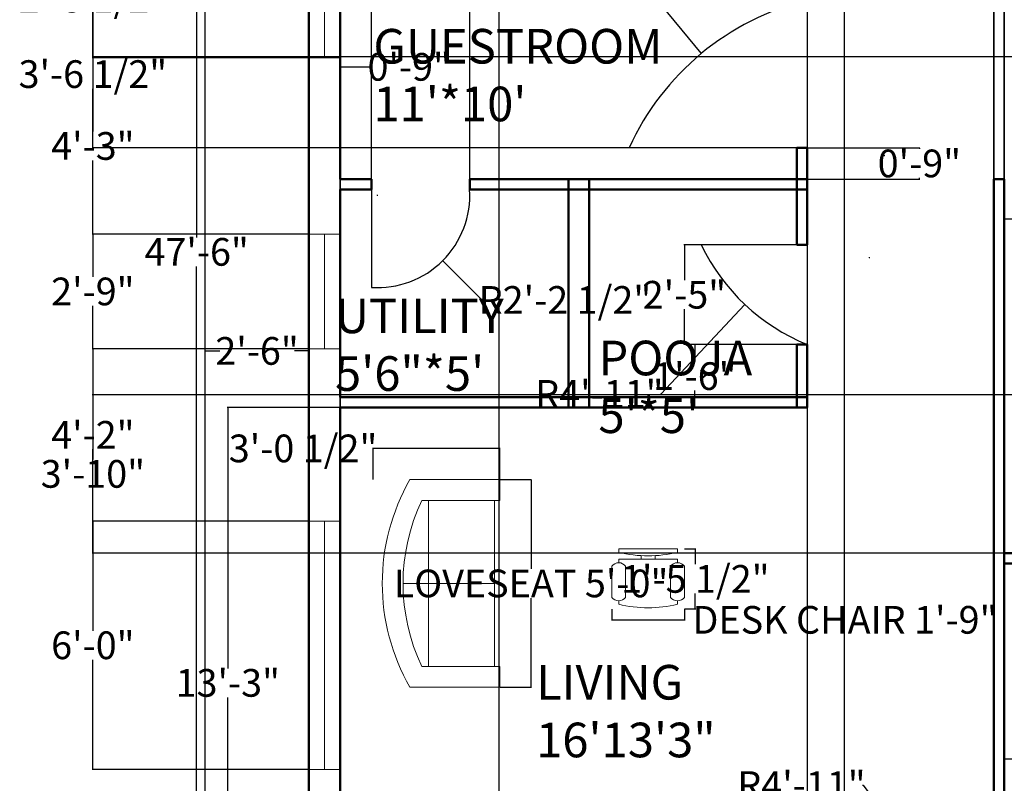
# Model space of a CAD drawing. Units: inches. Extents: x 3437 to 3994, y 3379 to 4084.
# Tile 2 of 6: x 3437 to 3722, y 3555 to 3776. Entities that reach past the tile are written whole.
import ezdxf

# ---------------------------------------------------------------- set-up
doc = ezdxf.new("R2010")
doc.units = ezdxf.units.IN
doc.header["$MEASUREMENT"] = 0
for name, color, linetype, lineweight in [('A-ANNO-DIMS', 2, 'Continuous', 18), ('A-AREA-IDEN', 7, 'Continuous', 25), ('A-DOOR', 3, 'Continuous', 25), ('A-FLOR-CASE', 8, 'Continuous', 25), ('A-FLOR-STRS', 7, 'Continuous', 25), ('A-FURN', 8, 'Continuous', 18), ('A-GLAZ', 4, 'Continuous', 18), ('A-WALL', 7, 'Continuous', 50), ('C-PROP', 3, 'Continuous', 25)]:
    doc.layers.add(name, color=color, linetype=linetype, lineweight=lineweight)
doc.styles.get("Standard").update_dxf_attribs({"font": 'arial.ttf'})
doc.dimstyles.get("Standard").update_dxf_attribs({"dimtxt": 8, "dimasz": 0.18, "dimexe": 0.18, "dimexo": 0.0625, "dimgap": 0.09, "dimtad": 0, "dimtih": 1, "dimtoh": 1, "dimdec": 0, "dimzin": 0, "dimdsep": 46, "dimlunit": 3, "dimtxsty": 'Standard', "dimcen": 0.09, "dimadec": 0, "dimazin": 0, "dimtfac": 1, "dimtdec": 0, "dimtofl": 0, "dimtmove": 0, "dimatfit": 3, "dimfxl": 1, "dimtolj": 1, "dimtzin": 0, "dimarcsym": 0})

# ---------------------------------------------------------------- blocks, each defined once
blk = doc.blocks.new('Sofa - Roundback Loveseat 5 ft.')
for p, q in [((0, -32.44198), (0, -5.99998)), ((-24, -33.99998), (-24, -11.46958)), ((-23.9998, -13.38178), (23.99986, -13.38178)), ((24.00004, -33.99998), (24.00004, -11.46958)), ((-24, -32.44198), (24.00004, -32.44198))]:
    blk.add_line(p, q)
for points in [[(-24, -33.99998), (-30, -33.99998), (-30, -7.99998)], [(30.00004, -7.99998), (30.00004, -33.99998), (24.00004, -33.99998)]]:
    blk.add_lwpolyline(points)
for centre, radius, start, end in [((0, -60.24998), 60.24998, 60.13715, 119.8628), ((0, -61.38438), 55.38444, 64.32083, 115.6792)]:
    blk.add_arc(centre, radius, start, end)
blk = doc.blocks.new('Chair - Desk')
for p, q in [((-8.5, 0), (-8.5, -1)), ((-8.5, 0), (8.5, 0)), ((8.5, 0), (8.5, -1)), ((-2, -3), (-2, -1.9355)), ((2, -1.9576), (2, -3)), ((-10.5, -5), (-10.5, -14)), ((-8.5, -3), (-8.5, -4)), ((-8.5, -3), (8.5, -3)), ((-6.5, -14), (-6.5, -5)), ((6.5, -5), (6.5, -14)), ((8.5, -3), (8.5, -4)), ((10.5, -14), (10.5, -5)), ((-8.5, -15), (-8.5, -16)), ((8.5, -15), (8.5, -16))]:
    blk.add_line(p, q)
for centre, radius, start, end in [((0, 34.625), 36.625, 256.5803, 283.4197), ((-8.5, -6.5), 2.5, 36.8699, 143.1301), ((8.5, -6.5), 2.5, 36.8699, 143.1301), ((-8.5, -12.5), 2.5, 216.8699, 323.1301), ((8.5, -12.5), 2.5, 216.8699, 323.1301), ((0, 19.625), 36.625, 256.5803, 283.4197)]:
    blk.add_arc(centre, radius, start, end)
blk = doc.blocks.new('*D12')
at = {"layer": 'A-ANNO-DIMS', "color": 0, "lineweight": -2, "transparency": 16777216}
for p, q in [((3491.02, 3671.63), (3491.02, 3680.21)), ((3491.2, 3680.03), (3495.23, 3680.03)), ((3520.84, 3680.03), (3516.82, 3680.03)), ((3521.02, 3671.63), (3521.02, 3680.21))]:
    blk.add_line(p, q, dxfattribs=at)
at = {"layer": 'A-ANNO-DIMS', "color": 0, "transparency": 16777216}
for points in [[(3491.2, 3680.06), (3491.2, 3680), (3491.02, 3680.03)], [(3520.84, 3680.06), (3520.84, 3680), (3521.02, 3680.03)]]:
    blk.add_solid(points, dxfattribs=at)
at = {"layer": 'Defpoints', "color": 0, "transparency": 16777216}
for p in [(3491.02, 3680.03), (3491.02, 3671.57), (3521.02, 3671.57)]:
    blk.add_point(p, dxfattribs=at)
at = {"layer": 'A-ANNO-DIMS', "color": 0, "transparency": 16777216, "insert": (3506.02, 3680.03), "char_height": 8, "attachment_point": 5}
blk.add_mtext('\\A1;2\'-6"', dxfattribs=at)
blk = doc.blocks.new('*D21')
at = {"layer": 'A-ANNO-DIMS', "color": 0, "lineweight": -2, "transparency": 16777216}
for p, q in [((3576.28, 3642.87), (3585.4, 3642.87)), ((3585.22, 3642.69), (3585.22, 3617.09)), ((3585.22, 3583.05), (3585.22, 3608.64)), ((3576.28, 3582.87), (3585.4, 3582.87))]:
    blk.add_line(p, q, dxfattribs=at)
at = {"layer": 'A-ANNO-DIMS', "color": 0, "transparency": 16777216}
for points in [[(3585.19, 3642.69), (3585.25, 3642.69), (3585.22, 3642.87)], [(3585.19, 3583.05), (3585.25, 3583.05), (3585.22, 3582.87)]]:
    blk.add_solid(points, dxfattribs=at)
at = {"layer": 'Defpoints', "color": 0, "transparency": 16777216}
for p in [(3576.22, 3642.87), (3585.22, 3642.87), (3576.22, 3582.87)]:
    blk.add_point(p, dxfattribs=at)
at = {"layer": 'A-ANNO-DIMS', "color": 0, "transparency": 16777216, "insert": (3585.22, 3612.87), "char_height": 8, "attachment_point": 5}
blk.add_mtext('\\A1;LOVESEAT 5\'-0"', dxfattribs=at)
blk = doc.blocks.new('*D22')
at = {"layer": 'A-ANNO-DIMS', "color": 0, "lineweight": -2, "transparency": 16777216}
for p, q in [((3539.55, 3651.87), (3539.37, 3651.87)), ((3539.55, 3642.93), (3539.55, 3652.05)), ((3576.04, 3651.87), (3539.73, 3651.87)), ((3576.22, 3642.93), (3576.22, 3652.05))]:
    blk.add_line(p, q, dxfattribs=at)
at = {"layer": 'A-ANNO-DIMS', "color": 0, "transparency": 16777216}
for points in [[(3539.73, 3651.9), (3539.73, 3651.84), (3539.55, 3651.87)], [(3576.04, 3651.9), (3576.04, 3651.84), (3576.22, 3651.87)]]:
    blk.add_solid(points, dxfattribs=at)
at = {"layer": 'Defpoints', "color": 0, "transparency": 16777216}
for p in [(3539.55, 3651.87), (3539.55, 3642.87), (3576.22, 3642.87)]:
    blk.add_point(p, dxfattribs=at)
at = {"layer": 'A-ANNO-DIMS', "color": 0, "transparency": 16777216, "insert": (3519.33, 3651.87), "char_height": 8, "attachment_point": 5}
blk.add_mtext('\\A1;3\'-0 1/2"', dxfattribs=at)
blk = doc.blocks.new('*D25')
at = {"layer": 'A-ANNO-DIMS', "color": 0, "lineweight": -2, "transparency": 16777216}
for p, q in [((3608.56, 3605.44), (3608.56, 3602.17)), ((3629.56, 3605.44), (3629.56, 3602.17)), ((3608.74, 3602.35), (3629.38, 3602.35)), ((3629.56, 3602.35), (3629.74, 3602.35))]:
    blk.add_line(p, q, dxfattribs=at)
at = {"layer": 'A-ANNO-DIMS', "color": 0, "transparency": 16777216}
for points in [[(3608.74, 3602.38), (3608.74, 3602.32), (3608.56, 3602.35)], [(3629.38, 3602.38), (3629.38, 3602.32), (3629.56, 3602.35)]]:
    blk.add_solid(points, dxfattribs=at)
at = {"layer": 'Defpoints', "color": 0, "transparency": 16777216}
for p in [(3608.56, 3605.5), (3629.56, 3605.5), (3629.56, 3602.35)]:
    blk.add_point(p, dxfattribs=at)
at = {"layer": 'A-ANNO-DIMS', "color": 0, "transparency": 16777216, "insert": (3675.97, 3602.35), "char_height": 8, "attachment_point": 5}
blk.add_mtext('\\A1;DESK CHAIR 1\'-9"', dxfattribs=at)
blk = doc.blocks.new('*D26')
at = {"layer": 'A-ANNO-DIMS', "color": 0, "lineweight": -2, "transparency": 16777216}
for p, q in [((3629.62, 3622.84), (3632.89, 3622.84)), ((3632.71, 3622.66), (3632.71, 3618.39)), ((3632.71, 3605.68), (3632.71, 3609.94)), ((3629.62, 3605.5), (3632.89, 3605.5))]:
    blk.add_line(p, q, dxfattribs=at)
at = {"layer": 'A-ANNO-DIMS', "color": 0, "transparency": 16777216}
for points in [[(3632.68, 3622.66), (3632.74, 3622.66), (3632.71, 3622.84)], [(3632.68, 3605.68), (3632.74, 3605.68), (3632.71, 3605.5)]]:
    blk.add_solid(points, dxfattribs=at)
at = {"layer": 'Defpoints', "color": 0, "transparency": 16777216}
for p in [(3629.56, 3622.84), (3632.71, 3622.84), (3629.56, 3605.5)]:
    blk.add_point(p, dxfattribs=at)
at = {"layer": 'A-ANNO-DIMS', "color": 0, "transparency": 16777216, "insert": (3632.71, 3614.17), "char_height": 8, "attachment_point": 5}
blk.add_mtext('\\A1;1\'-5 1/2"', dxfattribs=at)
blk = doc.blocks.new('*D28')
at = {"layer": 'A-ANNO-DIMS', "color": 0, "lineweight": -2, "transparency": 16777216}
for p, q in [((3520.96, 3993.64), (3488.39, 3993.64)), ((3488.57, 3993.46), (3488.57, 3712.81)), ((3488.57, 3423.82), (3488.57, 3704.46)), ((3520.96, 3423.64), (3488.39, 3423.64))]:
    blk.add_line(p, q, dxfattribs=at)
at = {"layer": 'A-ANNO-DIMS', "color": 0, "transparency": 16777216}
for points in [[(3488.54, 3993.46), (3488.6, 3993.46), (3488.57, 3993.64)], [(3488.54, 3423.82), (3488.6, 3423.82), (3488.57, 3423.64)]]:
    blk.add_solid(points, dxfattribs=at)
at = {"layer": 'Defpoints', "color": 0, "transparency": 16777216}
for p in [(3488.57, 3993.64), (3521.02, 3993.64), (3521.02, 3423.64)]:
    blk.add_point(p, dxfattribs=at)
at = {"layer": 'A-ANNO-DIMS', "color": 0, "transparency": 16777216, "insert": (3488.57, 3708.64), "char_height": 8, "attachment_point": 5}
blk.add_mtext('\\A1;47\'-6"', dxfattribs=at)
blk = doc.blocks.new('*D36')
at = {"layer": 'A-ANNO-DIMS', "color": 0, "lineweight": -2, "transparency": 16777216}
for p, q in [((3520.96, 3821.48), (3458.39, 3821.48)), ((3458.57, 3821.3), (3458.57, 3797.26)), ((3458.57, 3764.87), (3458.57, 3788.91)), ((3520.96, 3764.69), (3458.39, 3764.69))]:
    blk.add_line(p, q, dxfattribs=at)
at = {"layer": 'A-ANNO-DIMS', "color": 0, "transparency": 16777216}
for points in [[(3458.54, 3821.3), (3458.6, 3821.3), (3458.57, 3821.48)], [(3458.54, 3764.87), (3458.6, 3764.87), (3458.57, 3764.69)]]:
    blk.add_solid(points, dxfattribs=at)
at = {"layer": 'Defpoints', "color": 0, "transparency": 16777216}
for p in [(3521.02, 3821.48), (3458.57, 3764.69), (3521.02, 3764.69)]:
    blk.add_point(p, dxfattribs=at)
at = {"layer": 'A-ANNO-DIMS', "color": 0, "transparency": 16777216, "insert": (3458.57, 3793.09), "char_height": 8, "attachment_point": 5}
blk.add_mtext('\\A1;4\'-9"', dxfattribs=at)
blk = doc.blocks.new('*D37')
at = {"layer": 'A-ANNO-DIMS', "color": 0, "lineweight": -2, "transparency": 16777216}
for p, q in [((3520.96, 3764.69), (3458.39, 3764.69)), ((3458.57, 3764.51), (3458.57, 3743.41)), ((3458.57, 3713.95), (3458.57, 3735.05)), ((3520.96, 3713.77), (3458.39, 3713.77))]:
    blk.add_line(p, q, dxfattribs=at)
at = {"layer": 'A-ANNO-DIMS', "color": 0, "transparency": 16777216}
for points in [[(3458.54, 3764.51), (3458.6, 3764.51), (3458.57, 3764.69)], [(3458.54, 3713.95), (3458.6, 3713.95), (3458.57, 3713.77)]]:
    blk.add_solid(points, dxfattribs=at)
at = {"layer": 'Defpoints', "color": 0, "transparency": 16777216}
for p in [(3521.02, 3764.69), (3458.57, 3713.77), (3521.02, 3713.77)]:
    blk.add_point(p, dxfattribs=at)
at = {"layer": 'A-ANNO-DIMS', "color": 0, "transparency": 16777216, "insert": (3458.57, 3739.23), "char_height": 8, "attachment_point": 5}
blk.add_mtext('\\A1;4\'-3"', dxfattribs=at)
blk = doc.blocks.new('*D38')
at = {"layer": 'A-ANNO-DIMS', "color": 0, "lineweight": -2, "transparency": 16777216}
for p, q in [((3520.96, 3713.77), (3458.39, 3713.77)), ((3458.57, 3713.59), (3458.57, 3701.39)), ((3458.57, 3680.83), (3458.57, 3693.04)), ((3520.96, 3680.65), (3458.39, 3680.65))]:
    blk.add_line(p, q, dxfattribs=at)
at = {"layer": 'A-ANNO-DIMS', "color": 0, "transparency": 16777216}
for points in [[(3458.54, 3713.59), (3458.6, 3713.59), (3458.57, 3713.77)], [(3458.54, 3680.83), (3458.6, 3680.83), (3458.57, 3680.65)]]:
    blk.add_solid(points, dxfattribs=at)
at = {"layer": 'Defpoints', "color": 0, "transparency": 16777216}
for p in [(3521.02, 3713.77), (3458.57, 3680.65), (3521.02, 3680.65)]:
    blk.add_point(p, dxfattribs=at)
at = {"layer": 'A-ANNO-DIMS', "color": 0, "transparency": 16777216, "insert": (3458.57, 3697.21), "char_height": 8, "attachment_point": 5}
blk.add_mtext('\\A1;2\'-9"', dxfattribs=at)
blk = doc.blocks.new('*D39')
at = {"layer": 'A-ANNO-DIMS', "color": 0, "lineweight": -2, "transparency": 16777216}
for p, q in [((3520.96, 3680.65), (3458.39, 3680.65)), ((3458.57, 3680.47), (3458.57, 3659.88)), ((3458.57, 3631.08), (3458.57, 3651.67)), ((3520.96, 3630.9), (3458.39, 3630.9))]:
    blk.add_line(p, q, dxfattribs=at)
at = {"layer": 'A-ANNO-DIMS', "color": 0, "transparency": 16777216}
for points in [[(3458.54, 3680.47), (3458.6, 3680.47), (3458.57, 3680.65)], [(3458.54, 3631.08), (3458.6, 3631.08), (3458.57, 3630.9)]]:
    blk.add_solid(points, dxfattribs=at)
at = {"layer": 'Defpoints', "color": 0, "transparency": 16777216}
for p in [(3521.02, 3680.65), (3458.57, 3630.9), (3521.02, 3630.9)]:
    blk.add_point(p, dxfattribs=at)
at = {"layer": 'A-ANNO-DIMS', "color": 0, "transparency": 16777216, "insert": (3458.57, 3655.78), "char_height": 8, "attachment_point": 5}
blk.add_mtext('\\A1;4\'-2"', dxfattribs=at)
blk = doc.blocks.new('*D40')
at = {"layer": 'A-ANNO-DIMS', "color": 0, "lineweight": -2, "transparency": 16777216}
for p, q in [((3520.96, 3630.9), (3458.39, 3630.9)), ((3458.57, 3630.72), (3458.57, 3599.17)), ((3458.57, 3559.28), (3458.57, 3590.83)), ((3520.96, 3559.1), (3458.39, 3559.1))]:
    blk.add_line(p, q, dxfattribs=at)
at = {"layer": 'A-ANNO-DIMS', "color": 0, "transparency": 16777216}
for points in [[(3458.54, 3630.72), (3458.6, 3630.72), (3458.57, 3630.9)], [(3458.54, 3559.28), (3458.6, 3559.28), (3458.57, 3559.1)]]:
    blk.add_solid(points, dxfattribs=at)
at = {"layer": 'Defpoints', "color": 0, "transparency": 16777216}
for p in [(3521.02, 3630.9), (3458.57, 3559.1), (3521.02, 3559.1)]:
    blk.add_point(p, dxfattribs=at)
at = {"layer": 'A-ANNO-DIMS', "color": 0, "transparency": 16777216, "insert": (3458.57, 3595), "char_height": 8, "attachment_point": 5}
blk.add_mtext('\\A1;6\'-0"', dxfattribs=at)
blk = doc.blocks.new('*D46')
at = {"layer": 'A-ANNO-DIMS', "color": 0, "lineweight": -2, "transparency": 16777216}
for p, q in [((3576.02, 3426.7), (3576.02, 4056.27)), ((3576.2, 4056.09), (3635.57, 4056.09)), ((3721.84, 4056.09), (3662.48, 4056.09)), ((3722.02, 3426.7), (3722.02, 4056.27))]:
    blk.add_line(p, q, dxfattribs=at)
at = {"layer": 'A-ANNO-DIMS', "color": 0, "transparency": 16777216}
for points in [[(3576.2, 4056.12), (3576.2, 4056.06), (3576.02, 4056.09)], [(3721.84, 4056.12), (3721.84, 4056.06), (3722.02, 4056.09)]]:
    blk.add_solid(points, dxfattribs=at)
at = {"layer": 'Defpoints', "color": 0, "transparency": 16777216}
for p in [(3722.02, 4056.09), (3576.02, 3426.64), (3722.02, 3426.64)]:
    blk.add_point(p, dxfattribs=at)
at = {"layer": 'A-ANNO-DIMS', "color": 0, "transparency": 16777216, "insert": (3649.02, 4056.09), "char_height": 8, "attachment_point": 5}
blk.add_mtext('\\A1;12\'-2"', dxfattribs=at)
blk = doc.blocks.new('*D47')
at = {"layer": 'A-ANNO-DIMS', "color": 0, "lineweight": -2, "transparency": 16777216}
for p, q in [((3521.02, 3993.57), (3521.02, 3391.01)), ((3530.02, 3984.57), (3530.02, 3391.01)), ((3521.2, 3391.19), (3529.84, 3391.19)), ((3530.02, 3391.19), (3530.2, 3391.19))]:
    blk.add_line(p, q, dxfattribs=at)
at = {"layer": 'A-ANNO-DIMS', "color": 0, "transparency": 16777216}
for points in [[(3521.2, 3391.22), (3521.2, 3391.16), (3521.02, 3391.19)], [(3529.84, 3391.22), (3529.84, 3391.16), (3530.02, 3391.19)]]:
    blk.add_solid(points, dxfattribs=at)
at = {"layer": 'Defpoints', "color": 0, "transparency": 16777216}
for p in [(3521.02, 3993.64), (3530.02, 3984.64), (3530.02, 3391.19)]:
    blk.add_point(p, dxfattribs=at)
at = {"layer": 'A-ANNO-DIMS', "color": 0, "transparency": 16777216, "insert": (3540.93, 3391.19), "char_height": 8, "attachment_point": 5}
blk.add_mtext('\\A1;0\'-9"', dxfattribs=at)
blk = doc.blocks.new('*D48')
at = {"layer": 'A-ANNO-DIMS', "color": 0, "lineweight": -2, "transparency": 16777216}
for p, q in [((3722.02, 3861.57), (3722.02, 3391.01)), ((3719.02, 3858.57), (3719.02, 3391.01)), ((3719.2, 3391.19), (3721.84, 3391.19)), ((3722.02, 3391.19), (3722.2, 3391.19))]:
    blk.add_line(p, q, dxfattribs=at)
at = {"layer": 'A-ANNO-DIMS', "color": 0, "transparency": 16777216}
for points in [[(3719.2, 3391.22), (3719.2, 3391.16), (3719.02, 3391.19)], [(3721.84, 3391.22), (3721.84, 3391.16), (3722.02, 3391.19)]]:
    blk.add_solid(points, dxfattribs=at)
at = {"layer": 'Defpoints', "color": 0, "transparency": 16777216}
for p in [(3722.02, 3861.64), (3719.02, 3858.64), (3722.02, 3391.19)]:
    blk.add_point(p, dxfattribs=at)
at = {"layer": 'A-ANNO-DIMS', "color": 0, "transparency": 16777216, "insert": (3732.93, 3391.19), "char_height": 8, "attachment_point": 5}
blk.add_mtext('\\A1;0\'-3"', dxfattribs=at)
blk = doc.blocks.new('*D49')
at = {"layer": 'A-ANNO-DIMS', "color": 0, "lineweight": -2, "transparency": 16777216}
for p, q in [((3530.02, 3504.7), (3530.02, 4056.27)), ((3530.2, 4056.09), (3611.07, 4056.09)), ((3718.84, 4056.09), (3637.98, 4056.09)), ((3719.02, 3504.7), (3719.02, 4056.27))]:
    blk.add_line(p, q, dxfattribs=at)
at = {"layer": 'A-ANNO-DIMS', "color": 0, "transparency": 16777216}
for points in [[(3530.2, 4056.12), (3530.2, 4056.06), (3530.02, 4056.09)], [(3718.84, 4056.12), (3718.84, 4056.06), (3719.02, 4056.09)]]:
    blk.add_solid(points, dxfattribs=at)
at = {"layer": 'Defpoints', "color": 0, "transparency": 16777216}
for p in [(3719.02, 4056.09), (3530.02, 3504.64), (3719.02, 3504.64)]:
    blk.add_point(p, dxfattribs=at)
at = {"layer": 'A-ANNO-DIMS', "color": 0, "transparency": 16777216, "insert": (3624.52, 4056.09), "char_height": 8, "attachment_point": 5}
blk.add_mtext('\\A1;15\'-9"', dxfattribs=at)
blk = doc.blocks.new('*D50')
at = {"layer": 'A-ANNO-DIMS', "color": 0, "lineweight": -2, "transparency": 16777216}
for p, q in [((3529.96, 3663.64), (3497.39, 3663.64)), ((3497.57, 3663.46), (3497.57, 3588.31)), ((3497.57, 3504.82), (3497.57, 3579.96)), ((3529.96, 3504.64), (3497.39, 3504.64))]:
    blk.add_line(p, q, dxfattribs=at)
at = {"layer": 'A-ANNO-DIMS', "color": 0, "transparency": 16777216}
for points in [[(3497.54, 3663.46), (3497.6, 3663.46), (3497.57, 3663.64)], [(3497.54, 3504.82), (3497.6, 3504.82), (3497.57, 3504.64)]]:
    blk.add_solid(points, dxfattribs=at)
at = {"layer": 'Defpoints', "color": 0, "transparency": 16777216}
for p in [(3497.57, 3663.64), (3530.02, 3663.64), (3530.02, 3504.64)]:
    blk.add_point(p, dxfattribs=at)
at = {"layer": 'A-ANNO-DIMS', "color": 0, "transparency": 16777216, "insert": (3497.57, 3584.14), "char_height": 8, "attachment_point": 5}
blk.add_mtext('\\A1;13\'-3"', dxfattribs=at)
blk = doc.blocks.new('*D59')
at = {"layer": 'A-ANNO-DIMS', "color": 0, "lineweight": -2, "transparency": 16777216}
for p, q in [((3661.96, 3781.25), (3458.39, 3781.25)), ((3458.57, 3781.07), (3458.57, 3764.22)), ((3458.57, 3738.92), (3458.57, 3755.76)), ((3661.96, 3738.74), (3458.39, 3738.74))]:
    blk.add_line(p, q, dxfattribs=at)
at = {"layer": 'A-ANNO-DIMS', "color": 0, "transparency": 16777216}
for points in [[(3458.54, 3781.07), (3458.6, 3781.07), (3458.57, 3781.25)], [(3458.54, 3738.92), (3458.6, 3738.92), (3458.57, 3738.74)]]:
    blk.add_solid(points, dxfattribs=at)
at = {"layer": 'Defpoints', "color": 0, "transparency": 16777216}
for p in [(3662.02, 3781.25), (3458.57, 3738.74), (3662.02, 3738.74)]:
    blk.add_point(p, dxfattribs=at)
at = {"layer": 'A-ANNO-DIMS', "color": 0, "transparency": 16777216, "insert": (3458.57, 3759.99), "char_height": 8, "attachment_point": 5}
blk.add_mtext('\\A1;3\'-6 1/2"', dxfattribs=at)
blk = doc.blocks.new('*D60')
at = {"layer": 'A-ANNO-DIMS', "color": 0, "lineweight": -2, "transparency": 16777216}
for p, q in [((3539.11, 3729.7), (3539.11, 4056.27)), ((3539.29, 4056.09), (3567.31, 4056.09)), ((3567.49, 3729.7), (3567.49, 4056.27)), ((3567.49, 4056.09), (3567.67, 4056.09))]:
    blk.add_line(p, q, dxfattribs=at)
at = {"layer": 'A-ANNO-DIMS', "color": 0, "transparency": 16777216}
for points in [[(3539.29, 4056.12), (3539.29, 4056.06), (3539.11, 4056.09)], [(3567.31, 4056.12), (3567.31, 4056.06), (3567.49, 4056.09)]]:
    blk.add_solid(points, dxfattribs=at)
at = {"layer": 'Defpoints', "color": 0, "transparency": 16777216}
for p in [(3567.49, 4056.09), (3539.11, 3729.64), (3567.49, 3729.64)]:
    blk.add_point(p, dxfattribs=at)
at = {"layer": 'A-ANNO-DIMS', "color": 0, "transparency": 16777216, "insert": (3587.78, 4056.09), "char_height": 8, "attachment_point": 5}
blk.add_mtext('\\A1;2\'-4 1/2"', dxfattribs=at)
blk = doc.blocks.new('*D61')
at = {"layer": 'A-ANNO-DIMS', "color": 0, "lineweight": -2, "transparency": 16777216}
for p, q in [((3661.96, 3710.64), (3629.39, 3710.64)), ((3629.57, 3710.46), (3629.57, 3700.43)), ((3629.57, 3682.05), (3629.57, 3692.08)), ((3661.96, 3681.87), (3629.39, 3681.87))]:
    blk.add_line(p, q, dxfattribs=at)
at = {"layer": 'A-ANNO-DIMS', "color": 0, "transparency": 16777216}
for points in [[(3629.54, 3710.46), (3629.6, 3710.46), (3629.57, 3710.64)], [(3629.54, 3682.05), (3629.6, 3682.05), (3629.57, 3681.87)]]:
    blk.add_solid(points, dxfattribs=at)
at = {"layer": 'Defpoints', "color": 0, "transparency": 16777216}
for p in [(3629.57, 3710.64), (3662.02, 3710.64), (3662.02, 3681.87)]:
    blk.add_point(p, dxfattribs=at)
at = {"layer": 'A-ANNO-DIMS', "color": 0, "transparency": 16777216, "insert": (3629.57, 3696.25), "char_height": 8, "attachment_point": 5}
blk.add_mtext('\\A1;2\'-5"', dxfattribs=at)
blk = doc.blocks.new('*D66')
at = {"layer": 'A-ANNO-DIMS', "color": 0, "lineweight": -2, "transparency": 16777216}
for p, q in [((3871.96, 3667.39), (3458.39, 3667.39)), ((3458.57, 3667.21), (3458.57, 3648.69)), ((3458.57, 3621.82), (3458.57, 3640.34)), ((3871.96, 3621.64), (3458.39, 3621.64))]:
    blk.add_line(p, q, dxfattribs=at)
at = {"layer": 'A-ANNO-DIMS', "color": 0, "transparency": 16777216}
for points in [[(3458.54, 3667.21), (3458.6, 3667.21), (3458.57, 3667.39)], [(3458.54, 3621.82), (3458.6, 3621.82), (3458.57, 3621.64)]]:
    blk.add_solid(points, dxfattribs=at)
at = {"layer": 'Defpoints', "color": 0, "transparency": 16777216}
for p in [(3458.57, 3667.39), (3872.02, 3667.39), (3872.02, 3621.64)]:
    blk.add_point(p, dxfattribs=at)
at = {"layer": 'A-ANNO-DIMS', "color": 0, "transparency": 16777216, "insert": (3458.57, 3644.51), "char_height": 8, "attachment_point": 5}
blk.add_mtext('\\A1;3\'-10"', dxfattribs=at)
blk = doc.blocks.new('*D73')
at = {"layer": 'A-ANNO-DIMS', "color": 0, "lineweight": -2, "transparency": 16777216}
for p, q in [((3665.09, 3738.74), (3697.65, 3738.74)), ((3697.47, 3738.56), (3697.47, 3738.36)), ((3665.09, 3729.64), (3697.65, 3729.64)), ((3697.47, 3729.82), (3697.47, 3730.01))]:
    blk.add_line(p, q, dxfattribs=at)
at = {"layer": 'A-ANNO-DIMS', "color": 0, "transparency": 16777216}
for points in [[(3697.44, 3738.56), (3697.5, 3738.56), (3697.47, 3738.74)], [(3697.44, 3729.82), (3697.5, 3729.82), (3697.47, 3729.64)]]:
    blk.add_solid(points, dxfattribs=at)
at = {"layer": 'Defpoints', "color": 0, "transparency": 16777216}
for p in [(3665.02, 3738.74), (3665.02, 3729.64), (3697.47, 3729.64)]:
    blk.add_point(p, dxfattribs=at)
at = {"layer": 'A-ANNO-DIMS', "color": 0, "transparency": 16777216, "insert": (3697.47, 3734.19), "char_height": 8, "attachment_point": 5}
blk.add_mtext('\\A1;0\'-9"', dxfattribs=at)
blk = doc.blocks.new('*D74')
at = {"layer": 'A-ANNO-DIMS', "color": 0, "lineweight": -2, "transparency": 16777216}
for p, q in [((3530.02, 3729.7), (3530.02, 3762.27)), ((3530.2, 3762.09), (3538.93, 3762.09)), ((3539.11, 3729.7), (3539.11, 3762.27)), ((3539.11, 3762.09), (3539.29, 3762.09))]:
    blk.add_line(p, q, dxfattribs=at)
at = {"layer": 'A-ANNO-DIMS', "color": 0, "transparency": 16777216}
for points in [[(3530.2, 3762.12), (3530.2, 3762.06), (3530.02, 3762.09)], [(3538.93, 3762.12), (3538.93, 3762.06), (3539.11, 3762.09)]]:
    blk.add_solid(points, dxfattribs=at)
at = {"layer": 'Defpoints', "color": 0, "transparency": 16777216}
for p in [(3539.11, 3762.09), (3530.02, 3729.64), (3539.11, 3729.64)]:
    blk.add_point(p, dxfattribs=at)
at = {"layer": 'A-ANNO-DIMS', "color": 0, "transparency": 16777216, "insert": (3550.01, 3762.09), "char_height": 8, "attachment_point": 5}
blk.add_mtext('\\A1;0\'-9"', dxfattribs=at)
blk = doc.blocks.new('*D75')
at = {"layer": 'A-ANNO-DIMS', "color": 0, "lineweight": -2, "transparency": 16777216}
for p, q in [((3664.96, 3681.87), (3632.39, 3681.87)), ((3632.57, 3681.69), (3632.57, 3676.93)), ((3632.57, 3663.82), (3632.57, 3668.58)), ((3664.96, 3663.64), (3632.39, 3663.64))]:
    blk.add_line(p, q, dxfattribs=at)
at = {"layer": 'A-ANNO-DIMS', "color": 0, "transparency": 16777216}
for points in [[(3632.54, 3681.69), (3632.6, 3681.69), (3632.57, 3681.87)], [(3632.54, 3663.82), (3632.6, 3663.82), (3632.57, 3663.64)]]:
    blk.add_solid(points, dxfattribs=at)
at = {"layer": 'Defpoints', "color": 0, "transparency": 16777216}
for p in [(3632.57, 3681.87), (3665.02, 3681.87), (3665.02, 3663.64)]:
    blk.add_point(p, dxfattribs=at)
at = {"layer": 'A-ANNO-DIMS', "color": 0, "transparency": 16777216, "insert": (3632.57, 3672.75), "char_height": 8, "attachment_point": 5}
blk.add_mtext('\\A1;1\'-6"', dxfattribs=at)
blk = doc.blocks.new('*D79')
at = {"layer": 'A-ANNO-DIMS', "color": 0, "lineweight": -2, "transparency": 16777216}
for p, q in [((3675.76, 3905.25), (3675.76, 3391.01)), ((3665.02, 3903.57), (3665.02, 3391.01)), ((3665.2, 3391.19), (3675.58, 3391.19)), ((3675.76, 3391.19), (3675.94, 3391.19))]:
    blk.add_line(p, q, dxfattribs=at)
at = {"layer": 'A-ANNO-DIMS', "color": 0, "transparency": 16777216}
for points in [[(3665.2, 3391.22), (3665.2, 3391.16), (3665.02, 3391.19)], [(3675.58, 3391.22), (3675.58, 3391.16), (3675.76, 3391.19)]]:
    blk.add_solid(points, dxfattribs=at)
at = {"layer": 'Defpoints', "color": 0, "transparency": 16777216}
for p in [(3675.76, 3905.31), (3665.02, 3903.64), (3675.76, 3391.19)]:
    blk.add_point(p, dxfattribs=at)
at = {"layer": 'A-ANNO-DIMS', "color": 0, "transparency": 16777216, "insert": (3699.09, 3391.19), "char_height": 8, "attachment_point": 5}
blk.add_mtext('\\A1;0\'-10 1/2"', dxfattribs=at)
blk = doc.blocks.new('*D86')
at = {"layer": 'A-ANNO-DIMS', "color": 0, "lineweight": -2, "transparency": 16777216}
for p, q in [((3775.96, 3798.64), (3458.39, 3798.64)), ((3458.57, 3798.46), (3458.57, 3786.05)), ((3458.57, 3765.19), (3458.57, 3777.6)), ((3791.17, 3765.01), (3458.39, 3765.01))]:
    blk.add_line(p, q, dxfattribs=at)
at = {"layer": 'A-ANNO-DIMS', "color": 0, "transparency": 16777216}
for points in [[(3458.54, 3798.46), (3458.6, 3798.46), (3458.57, 3798.64)], [(3458.54, 3765.19), (3458.6, 3765.19), (3458.57, 3765.01)]]:
    blk.add_solid(points, dxfattribs=at)
at = {"layer": 'Defpoints', "color": 0, "transparency": 16777216}
for p in [(3776.02, 3798.64), (3458.57, 3765.01), (3791.23, 3765.01)]:
    blk.add_point(p, dxfattribs=at)
at = {"layer": 'A-ANNO-DIMS', "color": 0, "transparency": 16777216, "insert": (3458.57, 3781.82), "char_height": 8, "attachment_point": 5}
blk.add_mtext('\\A1;2\'-9 1/2"', dxfattribs=at)
blk = doc.blocks.new('*D87')
at = {"layer": 'A-ANNO-DIMS', "color": 0, "lineweight": -2, "transparency": 16777216}
for p, q in [((3605.04, 3801.24), (3605.22, 3801.24)), ((3605.22, 3801.24), (3634.29, 3766.05)), ((3682.97, 3707.03), (3683.15, 3707.03)), ((3683.06, 3706.94), (3683.06, 3707.12))]:
    blk.add_line(p, q, dxfattribs=at)
at = {"layer": 'A-ANNO-DIMS', "color": 0, "transparency": 16777216}
blk.add_solid([(3634.32, 3766.07), (3634.27, 3766.03), (3634.41, 3765.91)], dxfattribs=at)
at = {"layer": 'Defpoints', "color": 0, "transparency": 16777216}
for p in [(3634.41, 3765.91), (3683.06, 3707.03)]:
    blk.add_point(p, dxfattribs=at)
at = {"layer": 'A-ANNO-DIMS', "color": 0, "transparency": 16777216, "insert": (3581.17, 3801.24), "char_height": 8, "attachment_point": 5}
blk.add_mtext('\\A1;R6\'-4 1/2"', dxfattribs=at)
blk = doc.blocks.new('*D88')
at = {"layer": 'A-ANNO-DIMS', "color": 0, "lineweight": -2, "transparency": 16777216}
for p, q in [((3681.05, 3554.61), (3681.23, 3554.61)), ((3681.23, 3554.61), (3702.45, 3526.46)), ((3738.02, 3479.16), (3738.2, 3479.16)), ((3738.11, 3479.07), (3738.11, 3479.25))]:
    blk.add_line(p, q, dxfattribs=at)
at = {"layer": 'A-ANNO-DIMS', "color": 0, "transparency": 16777216}
blk.add_solid([(3702.48, 3526.48), (3702.43, 3526.44), (3702.56, 3526.32)], dxfattribs=at)
at = {"layer": 'Defpoints', "color": 0, "transparency": 16777216}
for p in [(3702.56, 3526.32), (3738.11, 3479.16)]:
    blk.add_point(p, dxfattribs=at)
at = {"layer": 'A-ANNO-DIMS', "color": 0, "transparency": 16777216, "insert": (3663.39, 3554.61), "char_height": 8, "attachment_point": 5}
blk.add_mtext('\\A1;R4\'-11"', dxfattribs=at)
blk = doc.blocks.new('*D89')
at = {"layer": 'A-ANNO-DIMS', "color": 0, "lineweight": -2, "transparency": 16777216}
for p, q in [((3687.35, 3736.47), (3687.53, 3736.47)), ((3687.44, 3736.38), (3687.44, 3736.56)), ((3622.81, 3667.61), (3646.92, 3693.3)), ((3622.63, 3667.61), (3622.81, 3667.61))]:
    blk.add_line(p, q, dxfattribs=at)
at = {"layer": 'A-ANNO-DIMS', "color": 0, "transparency": 16777216}
blk.add_solid([(3646.9, 3693.32), (3646.95, 3693.28), (3647.05, 3693.43)], dxfattribs=at)
at = {"layer": 'Defpoints', "color": 0, "transparency": 16777216}
for p in [(3687.44, 3736.47), (3647.05, 3693.43)]:
    blk.add_point(p, dxfattribs=at)
at = {"layer": 'A-ANNO-DIMS', "color": 0, "transparency": 16777216, "insert": (3604.97, 3667.61), "char_height": 8, "attachment_point": 5}
blk.add_mtext('\\A1;R4\'-11"', dxfattribs=at)
blk = doc.blocks.new('*D93')
at = {"layer": 'A-ANNO-DIMS', "color": 0, "lineweight": -2, "transparency": 16777216}
for p, q in [((3540.77, 3724.99), (3540.95, 3724.99)), ((3540.86, 3724.9), (3540.86, 3725.08)), ((3570.98, 3694.75), (3559.81, 3705.96)), ((3571.16, 3694.75), (3570.98, 3694.75))]:
    blk.add_line(p, q, dxfattribs=at)
at = {"layer": 'A-ANNO-DIMS', "color": 0, "transparency": 16777216}
blk.add_solid([(3559.83, 3705.99), (3559.79, 3705.94), (3559.68, 3706.09)], dxfattribs=at)
at = {"layer": 'Defpoints', "color": 0, "transparency": 16777216}
for p in [(3540.86, 3724.99), (3559.68, 3706.09)]:
    blk.add_point(p, dxfattribs=at)
at = {"layer": 'A-ANNO-DIMS', "color": 0, "transparency": 16777216, "insert": (3595.03, 3694.75), "char_height": 8, "attachment_point": 5}
blk.add_mtext('\\A1;R2\'-2 1/2"', dxfattribs=at)

msp = doc.modelspace()

# ---------------------------------------------------------------- linework, layer by layer
at = {"layer": 'A-DOOR'}
for p, q in [((3662.02, 3738.74), (3613.57, 3738.74)), ((3539.11, 3726.64), (3539.11, 3698.38)), ((3662.02, 3710.64), (3634.37, 3710.64))]:
    msp.add_line(p, q, dxfattribs=at)
for centre, radius, start, end in [((3683.06, 3707.03), 76.38, 103.6573, 155.4718), ((3540.86, 3724.99), 26.67, 266.2248, 3.5338), ((3687.44, 3736.47), 59.02, 205.9481, 247.679)]:
    msp.add_arc(centre, radius, start, end, dxfattribs=at)
at = {"layer": 'A-FLOR-CASE'}
msp.add_line((3722.02, 3718.21), (3758.54, 3718.21), dxfattribs=at)
at = {"layer": 'A-FLOR-STRS'}
msp.add_line((3757.11, 3562.1), (3722.02, 3562.1), dxfattribs=at)
at = {"layer": 'A-GLAZ'}
for p, q in [((3525.52, 3821.48), (3525.52, 3764.69)), ((3521.02, 3764.69), (3530.02, 3764.69)), ((3521.02, 3713.77), (3530.02, 3713.77)), ((3525.52, 3713.77), (3525.52, 3680.65)), ((3521.02, 3680.65), (3521.02, 3680.65)), ((3521.02, 3680.65), (3530.02, 3680.65)), ((3521.02, 3630.9), (3530.02, 3630.9)), ((3525.52, 3630.9), (3525.52, 3559.1)), ((3521.02, 3559.1), (3530.02, 3559.1))]:
    msp.add_line(p, q, dxfattribs=at)
at = {"layer": 'A-WALL'}
for p, q in [((3521.02, 3423.64), (3521.02, 3993.64)), ((3530.02, 3729.64), (3530.02, 3849.64)), ((3662.02, 3738.74), (3665.02, 3738.74)), ((3662.02, 3710.64), (3662.02, 3738.74)), ((3665.02, 3710.64), (3665.02, 3738.74)), ((3530.02, 3729.64), (3539.11, 3729.64)), ((3539.11, 3729.64), (3539.11, 3726.64)), ((3567.49, 3729.64), (3567.49, 3726.64)), ((3567.49, 3729.64), (3665.02, 3729.64)), ((3596.02, 3663.64), (3596.02, 3729.64)), ((3602.02, 3663.64), (3602.02, 3729.64)), ((3719.02, 3663.64), (3719.02, 3729.64)), ((3722.02, 3729.64), (3719.02, 3729.64)), ((3722.02, 3663.64), (3722.02, 3729.64)), ((3530.02, 3726.64), (3539.11, 3726.64)), ((3530.02, 3666.64), (3530.02, 3726.64)), ((3567.49, 3726.64), (3665.02, 3726.64)), ((3662.02, 3710.64), (3665.02, 3710.64)), ((3662.02, 3663.64), (3662.02, 3681.87)), ((3662.02, 3681.87), (3665.02, 3681.87)), ((3665.02, 3663.64), (3665.02, 3681.87)), ((3530.02, 3666.64), (3665.02, 3666.64)), ((3530.02, 3663.64), (3665.02, 3663.64)), ((3530.02, 3504.64), (3530.02, 3663.64)), ((3719.02, 3535.98), (3719.02, 3663.64)), ((3722.02, 3535.98), (3722.02, 3663.64)), ((3722.02, 3621.64), (3814.05, 3621.64)), ((3722.02, 3618.64), (3814.05, 3618.64))]:
    msp.add_line(p, q, dxfattribs=at)
at = {"layer": 'C-PROP'}
msp.add_lwpolyline([(3770.9, 3423.64), (3491.02, 3423.64), (3491.02, 4023.64), (3911.02, 4023.64), (3911.02, 3423.64), (3890.36, 3423.64)], dxfattribs=at)

# ---------------------------------------------------------------- block references
at = {"layer": 'A-FURN', "rotation": 90.0000150000014}
msp.add_blockref('Sofa - Roundback Loveseat 5 ft.', (3542.22, 3612.87), dxfattribs=at)
at = {"layer": 'A-FURN'}
msp.add_blockref('Chair - Desk', (3619.06, 3622.84), dxfattribs=at)

# ---------------------------------------------------------------- texts
at = {"layer": 'A-AREA-IDEN', "char_height": 10, "attachment_point": 1}
for s, insert in [("GUESTROOM\\P11'*10'", (3539.66, 3773.04)), ('UTILITY\\P5\'6"*5\'', (3528.55, 3695.16)), ("POOJA\\P5'*5'", (3604.7, 3682.98)), ('LIVING\\P16\'13\'3"', (3586.68, 3589.32))]:
    msp.add_mtext_dynamic_manual_height_columns(s, width=200.853, gutter_width=1, heights=[0], dxfattribs=dict(at, insert=insert))

# ---------------------------------------------------------------- dimensions: what is measured, and where the dimension line sits
at = {"layer": 'A-ANNO-DIMS'}
for base, p1, p2, override, picture, middle in [((3567.49, 4056.09), (3539.11, 3729.64), (3567.49, 3729.64), {"dimdec": 1, "dimlfac": 1, "dimrnd": 0, "dimzin": 1, "dimdsep": 46, "dimlunit": 4, "dimfrac": 2}, '*D60', (3587.78, 4056.09)), ((3719.02, 4056.09), (3530.02, 3504.64), (3719.02, 3504.64), {"dimdec": 1, "dimlfac": 1, "dimrnd": 0, "dimzin": 1, "dimdsep": 46, "dimlunit": 4, "dimfrac": 2}, '*D49', (3624.52, 4056.09)), ((3722.02, 4056.09), (3576.02, 3426.64), (3722.02, 3426.64), {"dimdec": 1, "dimlfac": 1, "dimrnd": 0, "dimzin": 1, "dimdsep": 46, "dimlunit": 4, "dimfrac": 2}, '*D46', (3649.02, 4056.09)), ((3530.02, 3391.19), (3521.02, 3993.64), (3530.02, 3984.64), {"dimdec": 1, "dimlfac": 1, "dimrnd": 0, "dimzin": 1, "dimdsep": 46, "dimlunit": 4, "dimfrac": 2}, '*D47', (3540.93, 3391.19)), ((3675.76, 3391.19), (3665.02, 3903.64), (3675.76, 3905.31), {"dimdec": 1, "dimlfac": 1, "dimrnd": 0, "dimzin": 1, "dimdsep": 46, "dimlunit": 4, "dimfrac": 2}, '*D79', (3699.09, 3391.19)), ((3722.02, 3391.19), (3719.02, 3858.64), (3722.02, 3861.64), {"dimdec": 1, "dimlfac": 1, "dimrnd": 0, "dimzin": 1, "dimdsep": 46, "dimlunit": 4, "dimfrac": 2}, '*D48', (3732.93, 3391.19)), ((3539.11, 3762.09), (3530.02, 3729.64), (3539.11, 3729.64), {"dimdec": 1, "dimlfac": 1, "dimrnd": 0, "dimzin": 1, "dimdsep": 46, "dimlunit": 4, "dimfrac": 2}, '*D74', (3550.01, 3762.09)), ((3491.02, 3680.03), (3521.02, 3671.57), (3491.02, 3671.57), {"dimclrd": 0, "dimclre": 0, "dimclrt": 0}, '*D12', (3506.02, 3680.03))]:
    dim = msp.add_linear_dim(base=base, p1=p1, p2=p2, dimstyle='Standard', override=override, dxfattribs=at)
    dim.commit()
    dim.dimension.update_dxf_attribs({"geometry": picture, "text_midpoint": middle})
for base, p1, p2, angle, picture, middle in [((3488.57, 3993.64), (3521.02, 3423.64), (3521.02, 3993.64), 90, '*D28', (3488.57, 3708.64)), ((3458.57, 3764.69), (3521.02, 3821.48), (3521.02, 3764.69), 90, '*D36', (3458.57, 3793.09)), ((3458.57, 3765.01), (3776.02, 3798.64), (3791.23, 3765.01), 90, '*D86', (3458.57, 3781.82)), ((3458.57, 3738.74), (3662.02, 3781.25), (3662.02, 3738.74), 90, '*D59', (3458.57, 3759.99)), ((3458.57, 3713.77), (3521.02, 3764.69), (3521.02, 3713.77), 90, '*D37', (3458.57, 3739.23)), ((3697.47, 3729.64), (3665.02, 3738.74), (3665.02, 3729.64), 270, '*D73', (3697.47, 3734.19)), ((3458.57, 3680.65), (3521.02, 3713.77), (3521.02, 3680.65), 90, '*D38', (3458.57, 3697.21)), ((3629.57, 3710.64), (3662.02, 3681.87), (3662.02, 3710.64), 90, '*D61', (3629.57, 3696.25)), ((3458.5743, 3630.901), (3521.0243, 3680.6541), (3521.0243, 3630.901), 90, '*D39', (3458.5743, 3655.7775)), ((3632.57, 3681.87), (3665.02, 3663.64), (3665.02, 3681.87), 90, '*D75', (3632.57, 3672.75)), ((3458.5743, 3667.394), (3872.0243, 3621.6359), (3872.0243, 3667.394), 90, '*D66', (3458.5743, 3644.515)), ((3497.57, 3663.64), (3530.02, 3504.64), (3530.02, 3663.64), 90, '*D50', (3497.57, 3584.14)), ((3539.55, 3651.87), (3576.22, 3642.87), (3539.55, 3642.87), 180, '*D22', (3519.33, 3651.87)), ((3458.57, 3559.1), (3521.02, 3630.9), (3521.02, 3559.1), 90, '*D40', (3458.57, 3595)), ((3632.71, 3622.84), (3629.56, 3605.5), (3629.56, 3622.84), 90, '*D26', (3632.71, 3614.17))]:
    dim = msp.add_linear_dim(base=base, p1=p1, p2=p2, angle=angle, dimstyle='Standard', override={"dimdec": 1, "dimlfac": 1, "dimrnd": 0, "dimzin": 1, "dimdsep": 46, "dimlunit": 4, "dimfrac": 2}, dxfattribs=at)
    dim.commit()
    dim.dimension.update_dxf_attribs({"geometry": picture, "text_midpoint": middle})
for center, mpoint, picture, middle in [((3683.06, 3707.03), (3634.41, 3765.91), '*D87', (3581.17, 3801.24)), ((3687.44, 3736.47), (3647.05, 3693.43), '*D89', (3604.97, 3667.61)), ((3540.86, 3724.99), (3559.68, 3706.09), '*D93', (3595.03, 3694.75)), ((3738.11, 3479.16), (3702.56, 3526.32), '*D88', (3663.39, 3554.61))]:
    dim = msp.add_radius_dim(center=center, mpoint=mpoint, dimstyle='Standard', override={"dimdec": 1, "dimlfac": 1, "dimrnd": 0, "dimzin": 1, "dimdsep": 46, "dimlunit": 4, "dimfrac": 2}, dxfattribs=at)
    dim.commit()
    dim.dimension.update_dxf_attribs({"geometry": picture, "text_midpoint": middle, "dimtype": 164})
dim = msp.add_linear_dim(base=(3585.22, 3642.87), p1=(3576.22, 3582.87), p2=(3576.22, 3642.87), angle=90, text='LOVESEAT <>', dimstyle='Standard', override={"dimdec": 1, "dimlfac": 1, "dimrnd": 0, "dimzin": 1, "dimdsep": 46, "dimlunit": 4, "dimfrac": 2}, dxfattribs=at)
dim.commit()
dim.dimension.update_dxf_attribs({"geometry": '*D21', "text_midpoint": (3585.22, 3612.87)})
dim = msp.add_linear_dim(base=(3629.56, 3602.35), p1=(3608.56, 3605.5), p2=(3629.56, 3605.5), text='DESK CHAIR <>', dimstyle='Standard', override={"dimdec": 1, "dimlfac": 1, "dimrnd": 0, "dimzin": 1, "dimdsep": 46, "dimlunit": 4, "dimfrac": 2}, dxfattribs=at)
dim.commit()
dim.dimension.update_dxf_attribs({"geometry": '*D25', "text_midpoint": (3675.97, 3602.35)})

doc.saveas('drawing.dxf')
